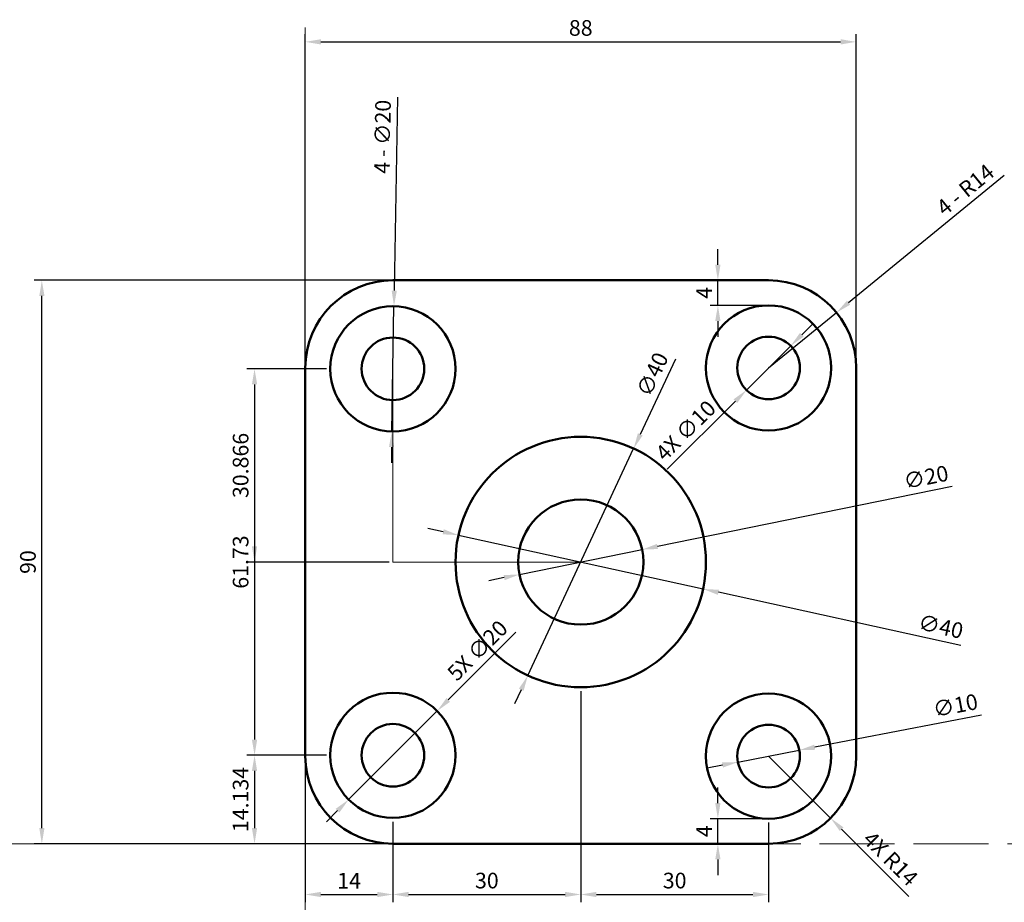
# Model space of a CAD drawing. Units: millimetres. Extents: x 3155 to 3312, y 1570 to 1711.
import ezdxf

# ---------------------------------------------------------------- set-up
doc = ezdxf.new("R2010")
doc.units = ezdxf.units.MM
doc.linetypes.add('ACAD_ISO02W100', pattern=[15, 12, -3])
doc.linetypes.add('CENTER', pattern=[50.8, 31.75, -6.35, 6.35, -6.35])
for name, color, linetype, lineweight in [('M-CNTR', 4, 'CENTER', 18), ('M-CONS', 8, 'ACAD_ISO02W100', 13), ('M-DIMS', 2, 'Continuous', 25), ('M-OUTL', 7, 'Continuous', 50)]:
    doc.layers.add(name, color=color, linetype=linetype, lineweight=lineweight)
doc.styles.get("Standard").update_dxf_attribs({"font": 'arial.ttf'})
doc.dimstyles.new('ISO-25', dxfattribs={"dimtxt": 2.5, "dimasz": 2.5, "dimexe": 1.25, "dimexo": 0.625, "dimtad": 1, "dimtxsty": 'Standard', "dimcen": 2.5, "dimadec": 0, "dimazin": 0, "dimtfac": 1, "dimtmove": 0, "dimatfit": 3, "dimfxl": 1, "dimarcsym": 0})

# ---------------------------------------------------------------- blocks, each defined once
blk = doc.blocks.new('*D1')
at = {"layer": 'Defpoints', "color": 0, "transparency": 16777216}
for p in [(3285.57, 1664.49), (3274.72, 1655.64)]:
    blk.add_point(p, dxfattribs=at)
at = {"layer": 'M-DIMS', "color": 0, "lineweight": -2, "transparency": 16777216}
for p, q in [((3312.37, 1686.36), (3287.51, 1666.07)), ((3274.72, 1655.64), (3285.57, 1664.49))]:
    blk.add_line(p, q, dxfattribs=at)
at = {"layer": 'M-DIMS', "color": 0, "transparency": 16777216}
blk.add_solid([(3287.24, 1666.39), (3287.77, 1665.75), (3285.57, 1664.49)], dxfattribs=at)
at = {"layer": 'M-DIMS', "color": 0, "transparency": 16777216, "insert": (3306.34, 1683.87), "char_height": 2.5, "attachment_point": 5, "rotation": 39.2108}
blk.add_mtext('4 - R14', dxfattribs=at)
blk = doc.blocks.new('*D2')
at = {"layer": 'Defpoints', "color": 0, "transparency": 16777216}
for p in [(3225.19, 1628.94), (3264.25, 1620.34)]:
    blk.add_point(p, dxfattribs=at)
at = {"layer": 'M-DIMS', "color": 0, "lineweight": -2, "transparency": 16777216}
for p, q in [((3222.75, 1629.47), (3220.31, 1630.01)), ((3225.19, 1628.94), (3264.25, 1620.34)), ((3305.42, 1611.29), (3266.7, 1619.81))]:
    blk.add_line(p, q, dxfattribs=at)
at = {"layer": 'M-DIMS', "color": 0, "transparency": 16777216}
for points in [[(3222.84, 1629.88), (3222.66, 1629.07), (3225.19, 1628.94)], [(3266.79, 1620.21), (3266.61, 1619.4), (3264.25, 1620.34)]]:
    blk.add_solid(points, dxfattribs=at)
at = {"layer": 'M-DIMS', "color": 0, "transparency": 16777216, "insert": (3302.16, 1614.03), "char_height": 2.5, "attachment_point": 5, "rotation": 347.596}
blk.add_mtext('∅40', dxfattribs=at)
blk = doc.blocks.new('*D3')
at = {"layer": 'Defpoints', "color": 0, "transparency": 16777216}
for p in [(3254.52, 1626.63), (3234.92, 1622.65)]:
    blk.add_point(p, dxfattribs=at)
at = {"layer": 'M-DIMS', "color": 0, "lineweight": -2, "transparency": 16777216}
for p, q in [((3304.02, 1636.7), (3256.97, 1627.13)), ((3234.92, 1622.65), (3254.52, 1626.63)), ((3232.47, 1622.15), (3230.02, 1621.65))]:
    blk.add_line(p, q, dxfattribs=at)
at = {"layer": 'M-DIMS', "color": 0, "transparency": 16777216}
for points in [[(3256.89, 1627.54), (3257.05, 1626.72), (3254.52, 1626.63)], [(3232.39, 1622.56), (3232.56, 1621.74), (3234.92, 1622.65)]]:
    blk.add_solid(points, dxfattribs=at)
at = {"layer": 'M-DIMS', "color": 0, "transparency": 16777216, "insert": (3299.93, 1637.88), "char_height": 2.5, "attachment_point": 5, "rotation": 11.4968}
blk.add_mtext('∅20', dxfattribs=at)
blk = doc.blocks.new('*D4')
at = {"layer": 'Defpoints', "color": 0, "transparency": 16777216}
for p in [(3214.89, 1665.51), (3214.55, 1645.51)]:
    blk.add_point(p, dxfattribs=at)
at = {"layer": 'M-DIMS', "color": 0, "lineweight": -2, "transparency": 16777216}
for p, q in [((3215.46, 1698.88), (3214.93, 1668)), ((3214.55, 1645.51), (3214.89, 1665.51)), ((3214.51, 1643.01), (3214.47, 1640.51))]:
    blk.add_line(p, q, dxfattribs=at)
at = {"layer": 'M-DIMS', "color": 0, "transparency": 16777216}
for points in [[(3214.52, 1668.01), (3215.35, 1668), (3214.89, 1665.51)], [(3214.09, 1643.02), (3214.92, 1643), (3214.55, 1645.51)]]:
    blk.add_solid(points, dxfattribs=at)
at = {"layer": 'M-DIMS', "color": 0, "transparency": 16777216, "insert": (3213.38, 1692.57), "char_height": 2.5, "attachment_point": 5, "rotation": 89.0225}
blk.add_mtext('4 - ∅20', dxfattribs=at)
blk = doc.blocks.new('*D5')
at = {"layer": 'Defpoints', "color": 0, "transparency": 16777216}
for p in [(3279.63, 1594.59), (3269.81, 1592.69)]:
    blk.add_point(p, dxfattribs=at)
at = {"layer": 'M-DIMS', "color": 0, "lineweight": -2, "transparency": 16777216}
for p, q in [((3308.7, 1600.2), (3282.09, 1595.06)), ((3269.81, 1592.69), (3279.63, 1594.59)), ((3267.36, 1592.22), (3264.9, 1591.74))]:
    blk.add_line(p, q, dxfattribs=at)
at = {"layer": 'M-DIMS', "color": 0, "transparency": 16777216}
for points in [[(3282.01, 1595.47), (3282.16, 1594.65), (3279.63, 1594.59)], [(3267.28, 1592.63), (3267.44, 1591.81), (3269.81, 1592.69)]]:
    blk.add_solid(points, dxfattribs=at)
at = {"layer": 'M-DIMS', "color": 0, "transparency": 16777216, "insert": (3304.62, 1601.42), "char_height": 2.5, "attachment_point": 5, "rotation": 10.9283}
blk.add_mtext('∅10', dxfattribs=at)
blk = doc.blocks.new('*D6')
at = {"layer": 'Defpoints', "color": 0, "transparency": 16777216}
for p in [(3158.65, 1669.64), (3244.72, 1669.64), (3244.72, 1579.64)]:
    blk.add_point(p, dxfattribs=at)
at = {"layer": 'M-DIMS', "color": 0, "lineweight": -2, "transparency": 16777216}
for p, q in [((3244.1, 1669.64), (3157.4, 1669.64)), ((3158.65, 1582.14), (3158.65, 1667.14)), ((3244.1, 1579.64), (3157.4, 1579.64))]:
    blk.add_line(p, q, dxfattribs=at)
at = {"layer": 'M-DIMS', "color": 0, "transparency": 16777216}
for points in [[(3158.24, 1667.14), (3159.07, 1667.14), (3158.65, 1669.64)], [(3158.24, 1582.14), (3159.07, 1582.14), (3158.65, 1579.64)]]:
    blk.add_solid(points, dxfattribs=at)
at = {"layer": 'M-DIMS', "color": 0, "transparency": 16777216, "insert": (3156.75, 1624.64), "char_height": 2.5, "attachment_point": 5, "rotation": 90}
blk.add_mtext('90', dxfattribs=at)
blk = doc.blocks.new('*D7')
at = {"layer": 'Defpoints', "color": 0, "transparency": 16777216}
for p in [(3288.72, 1707.73), (3200.72, 1624.64), (3288.72, 1624.64)]:
    blk.add_point(p, dxfattribs=at)
at = {"layer": 'M-DIMS', "color": 0, "lineweight": -2, "transparency": 16777216}
for p, q in [((3200.72, 1625.27), (3200.72, 1708.98)), ((3288.72, 1625.27), (3288.72, 1708.98)), ((3203.22, 1707.73), (3286.22, 1707.73))]:
    blk.add_line(p, q, dxfattribs=at)
at = {"layer": 'M-DIMS', "color": 0, "transparency": 16777216}
for points in [[(3203.22, 1708.15), (3203.22, 1707.31), (3200.72, 1707.73)], [(3286.22, 1708.15), (3286.22, 1707.31), (3288.72, 1707.73)]]:
    blk.add_solid(points, dxfattribs=at)
at = {"layer": 'M-DIMS', "color": 0, "transparency": 16777216, "insert": (3244.72, 1709.63), "char_height": 2.5, "attachment_point": 5}
blk.add_mtext('88', dxfattribs=at)
blk = doc.blocks.new('HOLE-D10-CBORE-D20')
for radius in [10, 5]:
    blk.add_circle((0, 0), radius)
blk = doc.blocks.new('*D9')
at = {"layer": 'Defpoints', "color": 0, "transparency": 16777216}
for p in [(3200.72, 1593.64), (3214.72, 1583.77), (3214.72, 1571.54)]:
    blk.add_point(p, dxfattribs=at)
at = {"layer": 'M-DIMS', "color": 0, "lineweight": -2, "transparency": 16777216}
for p, q in [((3200.72, 1593.02), (3200.72, 1570.29)), ((3214.72, 1583.15), (3214.72, 1570.29)), ((3203.22, 1571.54), (3212.22, 1571.54))]:
    blk.add_line(p, q, dxfattribs=at)
at = {"layer": 'M-DIMS', "color": 0, "transparency": 16777216}
for points in [[(3203.22, 1571.96), (3203.22, 1571.12), (3200.72, 1571.54)], [(3212.22, 1571.96), (3212.22, 1571.12), (3214.72, 1571.54)]]:
    blk.add_solid(points, dxfattribs=at)
at = {"layer": 'M-DIMS', "color": 0, "transparency": 16777216, "insert": (3207.72, 1573.42), "char_height": 2.5, "attachment_point": 5}
blk.add_mtext('14', dxfattribs=at)
blk = doc.blocks.new('*D10')
at = {"layer": 'Defpoints', "color": 0, "transparency": 16777216}
for p in [(3244.72, 1604.64), (3214.72, 1583.77), (3244.72, 1571.54)]:
    blk.add_point(p, dxfattribs=at)
at = {"layer": 'M-DIMS', "color": 0, "lineweight": -2, "transparency": 16777216}
for p, q in [((3244.72, 1604.02), (3244.72, 1570.29)), ((3214.72, 1583.15), (3214.72, 1570.29)), ((3217.22, 1571.54), (3242.22, 1571.54))]:
    blk.add_line(p, q, dxfattribs=at)
at = {"layer": 'M-DIMS', "color": 0, "transparency": 16777216}
for points in [[(3217.22, 1571.96), (3217.22, 1571.12), (3214.72, 1571.54)], [(3242.22, 1571.96), (3242.22, 1571.12), (3244.72, 1571.54)]]:
    blk.add_solid(points, dxfattribs=at)
at = {"layer": 'M-DIMS', "color": 0, "transparency": 16777216, "insert": (3229.72, 1573.44), "char_height": 2.5, "attachment_point": 5}
blk.add_mtext('30', dxfattribs=at)
blk = doc.blocks.new('*D11')
at = {"layer": 'Defpoints', "color": 0, "transparency": 16777216}
for p in [(3244.72, 1604.64), (3274.72, 1583.64), (3274.72, 1571.54)]:
    blk.add_point(p, dxfattribs=at)
at = {"layer": 'M-DIMS', "color": 0, "lineweight": -2, "transparency": 16777216}
for p, q in [((3244.72, 1604.02), (3244.72, 1570.29)), ((3274.72, 1583.02), (3274.72, 1570.29)), ((3247.22, 1571.54), (3272.22, 1571.54))]:
    blk.add_line(p, q, dxfattribs=at)
at = {"layer": 'M-DIMS', "color": 0, "transparency": 16777216}
for points in [[(3247.22, 1571.96), (3247.22, 1571.12), (3244.72, 1571.54)], [(3272.22, 1571.96), (3272.22, 1571.12), (3274.72, 1571.54)]]:
    blk.add_solid(points, dxfattribs=at)
at = {"layer": 'M-DIMS', "color": 0, "transparency": 16777216, "insert": (3259.72, 1573.44), "char_height": 2.5, "attachment_point": 5}
blk.add_mtext('30', dxfattribs=at)
blk = doc.blocks.new('*D12')
at = {"layer": 'Defpoints', "color": 0, "transparency": 16777216}
for p in [(3266.62, 1669.64), (3274.72, 1669.64), (3274.72, 1665.64)]:
    blk.add_point(p, dxfattribs=at)
at = {"layer": 'M-DIMS', "color": 0, "lineweight": -2, "transparency": 16777216}
for p, q in [((3266.62, 1672.14), (3266.62, 1674.64)), ((3274.1, 1669.64), (3265.37, 1669.64)), ((3266.62, 1665.64), (3266.62, 1669.64)), ((3274.1, 1665.64), (3265.37, 1665.64)), ((3266.62, 1663.14), (3266.62, 1660.64))]:
    blk.add_line(p, q, dxfattribs=at)
at = {"layer": 'M-DIMS', "color": 0, "transparency": 16777216}
for points in [[(3266.2, 1672.14), (3267.04, 1672.14), (3266.62, 1669.64)], [(3266.2, 1663.14), (3267.04, 1663.14), (3266.62, 1665.64)]]:
    blk.add_solid(points, dxfattribs=at)
at = {"layer": 'M-DIMS', "color": 0, "transparency": 16777216, "insert": (3264.75, 1667.64), "char_height": 2.5, "attachment_point": 5, "rotation": 90}
blk.add_mtext('4', dxfattribs=at)
blk = doc.blocks.new('*D13')
at = {"layer": 'Defpoints', "color": 0, "transparency": 16777216}
for p in [(3266.62, 1583.64), (3274.72, 1583.64), (3274.72, 1579.64)]:
    blk.add_point(p, dxfattribs=at)
at = {"layer": 'M-DIMS', "color": 0, "lineweight": -2, "transparency": 16777216}
for p, q in [((3266.62, 1586.14), (3266.62, 1588.64)), ((3274.1, 1583.64), (3265.37, 1583.64)), ((3266.62, 1579.64), (3266.62, 1583.64)), ((3274.1, 1579.64), (3265.37, 1579.64)), ((3266.62, 1577.14), (3266.62, 1574.64))]:
    blk.add_line(p, q, dxfattribs=at)
at = {"layer": 'M-DIMS', "color": 0, "transparency": 16777216}
for points in [[(3266.2, 1586.14), (3267.04, 1586.14), (3266.62, 1583.64)], [(3266.2, 1577.14), (3267.04, 1577.14), (3266.62, 1579.64)]]:
    blk.add_solid(points, dxfattribs=at)
at = {"layer": 'M-DIMS', "color": 0, "transparency": 16777216, "insert": (3264.75, 1581.64), "char_height": 2.5, "attachment_point": 5, "rotation": 90}
blk.add_mtext('4', dxfattribs=at)
blk = doc.blocks.new('*D14')
at = {"layer": 'Defpoints', "color": 0, "transparency": 16777216}
for p in [(3204.72, 1655.51), (3192.62, 1593.77), (3204.72, 1593.77)]:
    blk.add_point(p, dxfattribs=at)
at = {"layer": 'M-DIMS', "color": 0, "lineweight": -2, "transparency": 16777216}
for p, q in [((3204.1, 1655.51), (3191.37, 1655.51)), ((3192.62, 1653.01), (3192.62, 1596.27)), ((3204.1, 1593.77), (3191.37, 1593.77))]:
    blk.add_line(p, q, dxfattribs=at)
at = {"layer": 'M-DIMS', "color": 0, "transparency": 16777216}
for points in [[(3192.2, 1653.01), (3193.04, 1653.01), (3192.62, 1655.51)], [(3192.2, 1596.27), (3193.04, 1596.27), (3192.62, 1593.77)]]:
    blk.add_solid(points, dxfattribs=at)
at = {"layer": 'M-DIMS', "color": 0, "transparency": 16777216, "insert": (3190.72, 1624.64), "char_height": 2.5, "attachment_point": 5, "rotation": 90}
blk.add_mtext('61.73', dxfattribs=at)
blk = doc.blocks.new('*D15')
at = {"layer": 'Defpoints', "color": 0, "transparency": 16777216}
for p in [(3204.72, 1593.77), (3192.62, 1579.64), (3214.72, 1579.64)]:
    blk.add_point(p, dxfattribs=at)
at = {"layer": 'M-DIMS', "color": 0, "lineweight": -2, "transparency": 16777216}
for p, q in [((3204.1, 1593.77), (3191.37, 1593.77)), ((3192.62, 1591.27), (3192.62, 1582.14)), ((3214.1, 1579.64), (3191.37, 1579.64))]:
    blk.add_line(p, q, dxfattribs=at)
at = {"layer": 'M-DIMS', "color": 0, "transparency": 16777216}
for points in [[(3192.2, 1591.27), (3193.04, 1591.27), (3192.62, 1593.77)], [(3192.2, 1582.14), (3193.04, 1582.14), (3192.62, 1579.64)]]:
    blk.add_solid(points, dxfattribs=at)
at = {"layer": 'M-DIMS', "color": 0, "transparency": 16777216, "insert": (3190.72, 1586.71), "char_height": 2.5, "attachment_point": 5, "rotation": 90}
blk.add_mtext('14.134', dxfattribs=at)
blk = doc.blocks.new('*D16')
at = {"layer": 'Defpoints', "color": 0, "transparency": 16777216}
for p in [(3204.72, 1655.51), (3192.62, 1624.64), (3214.72, 1624.64)]:
    blk.add_point(p, dxfattribs=at)
at = {"layer": 'M-DIMS', "color": 0, "lineweight": -2, "transparency": 16777216}
for p, q in [((3204.1, 1655.51), (3191.37, 1655.51)), ((3192.62, 1653.01), (3192.62, 1627.14)), ((3214.1, 1624.64), (3191.37, 1624.64))]:
    blk.add_line(p, q, dxfattribs=at)
at = {"layer": 'M-DIMS', "color": 0, "transparency": 16777216}
for points in [[(3192.2, 1653.01), (3193.04, 1653.01), (3192.62, 1655.51)], [(3192.2, 1627.14), (3193.04, 1627.14), (3192.62, 1624.64)]]:
    blk.add_solid(points, dxfattribs=at)
at = {"layer": 'M-DIMS', "color": 0, "transparency": 16777216, "insert": (3190.72, 1640.07), "char_height": 2.5, "attachment_point": 5, "rotation": 90}
blk.add_mtext('30.866', dxfattribs=at)
blk = doc.blocks.new('*D17')
at = {"layer": 'Defpoints', "color": 0, "transparency": 16777216}
for p in [(3253.17, 1642.77), (3236.27, 1606.51)]:
    blk.add_point(p, dxfattribs=at)
at = {"layer": 'M-DIMS', "color": 0, "lineweight": -2, "transparency": 16777216}
for p, q in [((3259.84, 1657.06), (3254.23, 1645.03)), ((3236.27, 1606.51), (3253.17, 1642.77)), ((3235.21, 1604.25), (3234.16, 1601.98))]:
    blk.add_line(p, q, dxfattribs=at)
at = {"layer": 'M-DIMS', "color": 0, "transparency": 16777216}
for points in [[(3253.85, 1645.21), (3254.61, 1644.86), (3253.17, 1642.77)], [(3234.84, 1604.42), (3235.59, 1604.07), (3236.27, 1606.51)]]:
    blk.add_solid(points, dxfattribs=at)
at = {"layer": 'M-DIMS', "color": 0, "transparency": 16777216, "insert": (3256.46, 1654.48), "char_height": 2.5, "attachment_point": 5, "rotation": 65.0038}
blk.add_mtext('∅40', dxfattribs=at)
blk = doc.blocks.new('*D18')
at = {"layer": 'Defpoints', "color": 0, "transparency": 16777216}
for p in [(3274.72, 1593.64), (3284.62, 1583.74)]:
    blk.add_point(p, dxfattribs=at)
at = {"layer": 'M-DIMS', "color": 0, "lineweight": -2, "transparency": 16777216}
for p, q in [((3274.72, 1593.64), (3284.62, 1583.74)), ((3297.12, 1571.23), (3286.39, 1581.97))]:
    blk.add_line(p, q, dxfattribs=at)
at = {"layer": 'M-DIMS', "color": 0, "transparency": 16777216}
blk.add_solid([(3286.68, 1582.27), (3286.09, 1581.68), (3284.62, 1583.74)], dxfattribs=at)
at = {"layer": 'M-DIMS', "color": 0, "transparency": 16777216, "insert": (3293.97, 1577.05), "char_height": 2.5, "attachment_point": 5, "rotation": 314.9942}
blk.add_mtext('4X R14', dxfattribs=at)
blk = doc.blocks.new('*D19')
at = {"layer": 'Defpoints', "color": 0, "transparency": 16777216}
for p in [(3221.79, 1600.85), (3207.65, 1586.7)]:
    blk.add_point(p, dxfattribs=at)
at = {"layer": 'M-DIMS', "color": 0, "lineweight": -2, "transparency": 16777216}
for p, q in [((3234.37, 1613.42), (3223.56, 1602.61)), ((3207.65, 1586.7), (3221.79, 1600.85)), ((3205.88, 1584.94), (3204.11, 1583.17))]:
    blk.add_line(p, q, dxfattribs=at)
at = {"layer": 'M-DIMS', "color": 0, "transparency": 16777216}
for points in [[(3223.27, 1602.91), (3223.85, 1602.32), (3221.79, 1600.85)], [(3205.59, 1585.23), (3206.18, 1584.64), (3207.65, 1586.7)]]:
    blk.add_solid(points, dxfattribs=at)
at = {"layer": 'M-DIMS', "color": 0, "transparency": 16777216, "insert": (3228.45, 1610.29), "char_height": 2.5, "attachment_point": 5, "rotation": 45.0004}
blk.add_mtext('5X ∅20', dxfattribs=at)
blk = doc.blocks.new('*D20')
at = {"layer": 'Defpoints', "color": 0, "transparency": 16777216}
for p in [(3278.26, 1659.18), (3271.19, 1652.11)]:
    blk.add_point(p, dxfattribs=at)
at = {"layer": 'M-DIMS', "color": 0, "lineweight": -2, "transparency": 16777216}
for p, q in [((3280.03, 1660.94), (3281.79, 1662.71)), ((3278.26, 1659.18), (3271.19, 1652.11)), ((3258.54, 1639.46), (3269.42, 1650.34))]:
    blk.add_line(p, q, dxfattribs=at)
at = {"layer": 'M-DIMS', "color": 0, "transparency": 16777216}
for points in [[(3279.73, 1661.24), (3280.32, 1660.65), (3278.26, 1659.18)], [(3269.12, 1650.63), (3269.71, 1650.04), (3271.19, 1652.11)]]:
    blk.add_solid(points, dxfattribs=at)
at = {"layer": 'M-DIMS', "color": 0, "transparency": 16777216, "insert": (3261.7, 1645.41), "char_height": 2.5, "attachment_point": 5, "rotation": 44.9922}
blk.add_mtext('4X ∅10', dxfattribs=at)

msp = doc.modelspace()

# ---------------------------------------------------------------- linework, layer by layer
at = {"layer": 'M-CNTR'}
for p, q in [((3214.7215, 1624.6405), (3214.7215, 1655.6405)), ((3244.7215, 1624.6405), (3214.7215, 1624.6405))]:
    msp.add_line(p, q, dxfattribs=at)
at = {"layer": 'M-CONS'}
for direction in [(0, 1), (1, 0)]:
    msp.add_xline((3200.7215, 1579.6405), direction, dxfattribs=at)
at = {"layer": 'M-OUTL'}
msp.add_lwpolyline([(3214.7215, 1579.6405), (3274.7215, 1579.6405, 0.41421356), (3288.7215, 1593.6405), (3288.7215, 1655.6405, 0.41421356), (3274.7215, 1669.6405), (3214.7215, 1669.6405, 0.41421356), (3200.7215, 1655.6405), (3200.7215, 1593.6405, 0.41421356)], format="xyb", close=True, dxfattribs=at)
for radius in [20, 10]:
    msp.add_circle((3244.7215, 1624.6405), radius, dxfattribs=at)

# ---------------------------------------------------------------- block references
for p in [(3214.7215, 1655.5067), (3274.7215, 1655.6405), (3214.7215, 1593.7744), (3274.7215, 1593.6405)]:
    msp.add_blockref('HOLE-D10-CBORE-D20', p, dxfattribs=at)

# ---------------------------------------------------------------- dimensions: what is measured, and where the dimension line sits
at = {"layer": 'M-DIMS'}
for base, p1, p2, override, picture, middle in [((3288.7215, 1707.7293), (3200.7215, 1624.6405), (3288.7215, 1624.6405), {"dimclrd": 0, "dimclre": 0, "dimclrt": 0}, '*D7', (3244.7215, 1709.6307)), ((3244.7215, 1571.5405), (3214.7215, 1583.7744), (3244.7215, 1604.6405), {"dimdec": 0, "dimlfac": 1, "dimrnd": 0, "dimzin": 0, "dimdsep": 46, "dimlunit": 2}, '*D10', (3229.7215, 1573.4428)), ((3274.7215, 1571.5405), (3244.7215, 1604.6405), (3274.7215, 1583.6405), {"dimdec": 0, "dimlfac": 1, "dimrnd": 0, "dimzin": 0, "dimdsep": 46, "dimlunit": 2}, '*D11', (3259.7215, 1573.4428)), ((3214.7215, 1571.5405), (3200.7215, 1593.6405), (3214.7215, 1583.7744), {"dimdec": 0, "dimlfac": 1, "dimrnd": 0, "dimzin": 0, "dimdsep": 46, "dimlunit": 2}, '*D9', (3207.7215, 1573.4206))]:
    dim = msp.add_linear_dim(base=base, p1=p1, p2=p2, dimstyle='ISO-25', override=override, dxfattribs=at)
    dim.commit()
    dim.dimension.update_dxf_attribs({"geometry": picture, "text_midpoint": middle})
for p1, p2, text, override, picture, middle in [((3214.5509, 1645.5081), (3214.8921, 1665.5052), '4 - <>', {"dimclrd": 0, "dimclre": 0, "dimclrt": 0}, '*D4', (3215.3533, 1692.5372)), ((3207.6505, 1586.7033), (3221.7925, 1600.8455), '5X <>', {"dimdec": 0, "dimlfac": 1, "dimrnd": 0, "dimzin": 0, "dimdsep": 46, "dimlunit": 2}, '*D19', (3229.8469, 1608.9))]:
    dim = msp.add_diameter_dim_2p(p1=p1, p2=p2, text=text, dimstyle='ISO-25', override=override, dxfattribs=at)
    dim.commit()
    dim.dimension.update_dxf_attribs({"geometry": picture, "text_midpoint": middle, "dimtype": 163})
dim = msp.add_radius_dim(center=(3274.7215, 1655.6405), mpoint=(3285.569, 1664.491), text='4 - <>', dimstyle='ISO-25', override={"dimclrd": 0, "dimclre": 0, "dimclrt": 0}, dxfattribs=at)
dim.commit()
dim.dimension.update_dxf_attribs({"geometry": '*D1', "text_midpoint": (3307.5305, 1682.4092), "dimtype": 164})
for base, p1, p2, override, picture, middle in [((3266.6215, 1669.6405), (3274.7215, 1665.6405), (3274.7215, 1669.6405), {"dimdec": 0, "dimlfac": 1, "dimrnd": 0, "dimzin": 0, "dimdsep": 46, "dimlunit": 2}, '*D12', (3264.7465, 1667.6405)), ((3158.6533, 1669.6405), (3244.7215, 1579.6405), (3244.7215, 1669.6405), {"dimclrd": 0, "dimclre": 0, "dimclrt": 0}, '*D6', (3156.7519, 1624.6405)), ((3192.6215, 1593.7744), (3204.7215, 1655.5067), (3204.7215, 1593.7744), {"dimdec": 2, "dimlfac": 1, "dimrnd": 0, "dimzin": 0, "dimdsep": 46, "dimlunit": 2}, '*D14', (3190.7192, 1624.6405)), ((3192.6215, 1624.6405), (3204.7215, 1655.5067), (3214.7215, 1624.6405), {"dimdec": 3, "dimlfac": 1, "dimrnd": 0, "dimzin": 0, "dimdsep": 46, "dimlunit": 2}, '*D16', (3190.7192, 1640.0736)), ((3192.6215, 1579.6405), (3204.7215, 1593.7744), (3214.7215, 1579.6405), {"dimdec": 3, "dimlfac": 1, "dimrnd": 0, "dimzin": 0, "dimdsep": 46, "dimlunit": 2}, '*D15', (3190.7192, 1586.7074)), ((3266.6215, 1583.6405), (3274.7215, 1579.6405), (3274.7215, 1583.6405), {"dimdec": 0, "dimlfac": 1, "dimrnd": 0, "dimzin": 0, "dimdsep": 46, "dimlunit": 2}, '*D13', (3264.7465, 1581.6405))]:
    dim = msp.add_linear_dim(base=base, p1=p1, p2=p2, angle=90, dimstyle='ISO-25', override=override, dxfattribs=at)
    dim.commit()
    dim.dimension.update_dxf_attribs({"geometry": picture, "text_midpoint": middle})
dim = msp.add_diameter_dim_2p(p1=(3278.2575, 1659.1756), p2=(3271.1855, 1652.1055), text='4X <>', dimstyle='ISO-25', override={"dimdec": 0, "dimlfac": 1, "dimrnd": 0, "dimzin": 0, "dimdsep": 46, "dimlunit": 2}, dxfattribs=at)
dim.commit()
dim.dimension.update_dxf_attribs({"geometry": '*D20', "text_midpoint": (3263.0944, 1644.0166)})
for p1, p2, override, picture, middle in [((3236.2703, 1606.5138), (3253.1726, 1642.7672), {"dimdec": 0, "dimlfac": 1, "dimrnd": 0, "dimzin": 0, "dimdsep": 46, "dimlunit": 2}, '*D17', (3258.2433, 1653.6433)), ((3234.9221, 1622.6474), (3254.5208, 1626.6336), {"dimclrd": 0, "dimclre": 0, "dimclrt": 0}, '*D3', (3300.3254, 1635.95)), ((3225.1883, 1628.9366), (3264.2546, 1620.3444), {"dimclrd": 0, "dimclre": 0, "dimclrt": 0}, '*D2', (3301.7375, 1612.1005)), ((3269.8122, 1592.6926), (3279.6308, 1594.5884), {"dimclrd": 0, "dimclre": 0, "dimclrt": 0}, '*D5', (3304.9964, 1599.4861))]:
    dim = msp.add_diameter_dim_2p(p1=p1, p2=p2, dimstyle='ISO-25', override=override, dxfattribs=at)
    dim.commit()
    dim.dimension.update_dxf_attribs({"geometry": picture, "text_midpoint": middle, "dimtype": 163})
dim = msp.add_radius_dim(center=(3274.7215, 1593.6405), mpoint=(3284.62, 1583.74), text='4X <>', dimstyle='ISO-25', override={"dimdec": 0, "dimlfac": 1, "dimrnd": 0, "dimzin": 0, "dimdsep": 46, "dimlunit": 2}, dxfattribs=at)
dim.commit()
dim.dimension.update_dxf_attribs({"geometry": '*D18', "text_midpoint": (3293.97, 1577.0485)})

doc.saveas('drawing.dxf')
